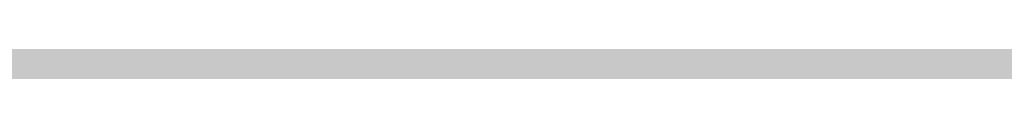
# Model space of a CAD drawing. Units: inches. Extents: x 2083 to 3317, y 1141 to 2115.
# Tile 151 of 256: x 3126.946713 to 3126.955939, y 1263.261503 to 1263.261646. Entities that reach past the tile are written whole.
import ezdxf

# ---------------------------------------------------------------- set-up
doc = ezdxf.new("R2010")
doc.units = ezdxf.units.IN
doc.layers.add('A-ANNO-DIMS', color=2, linetype='Continuous', lineweight=18)
doc.layers.add('A-WALL-PATT', color=251, linetype='Continuous', lineweight=13, true_color=0x636466)
doc.styles.get("Standard").update_dxf_attribs({"font": 'arial.ttf'})
doc.dimstyles.new('ISO-25', dxfattribs={"dimtxt": 12, "dimasz": 12, "dimexe": 1.25, "dimexo": 0.625, "dimtad": 1, "dimlunit": 3, "dimtxsty": 'Standard', "dimcen": 2.5, "dimadec": 0, "dimazin": 0, "dimtfac": 1, "dimtmove": 0, "dimatfit": 3, "dimfxl": 1, "dimarcsym": 0})

# ---------------------------------------------------------------- blocks, each defined once
blk = doc.blocks.new('*D26')
at = {"layer": 'A-ANNO-DIMS', "color": 0, "lineweight": -2, "transparency": 16777216}
for p, q in [((3088.985844, 1274.915092), (3088.985844, 1270.9519631)), ((3111.2400366, 1274.915092), (3111.2400366, 1270.9519631)), ((3076.985844, 1272.2019631), (2840.262447, 1272.2019631)), ((3111.2400366, 1272.2019631), (3088.985844, 1272.2019631)), ((3123.2400366, 1272.2019631), (3135.2400366, 1272.2019631))]:
    blk.add_line(p, q, dxfattribs=at)
at = {"layer": 'A-ANNO-DIMS', "color": 0, "transparency": 16777216}
for points in [[(3076.985844, 1274.2019631), (3076.985844, 1270.2019631), (3088.985844, 1272.2019631)], [(3123.2400366, 1274.2019631), (3123.2400366, 1270.2019631), (3111.2400366, 1272.2019631)]]:
    blk.add_solid(points, dxfattribs=at)
at = {"layer": 'Defpoints', "color": 0, "transparency": 16777216}
for p in [(3088.985844, 1275.540092), (3111.2400366, 1275.540092), (3088.985844, 1272.2019631)]:
    blk.add_point(p, dxfattribs=at)
at = {"layer": 'A-ANNO-DIMS', "color": 0, "transparency": 16777216, "insert": (2952.6241455, 1279.0316016), "char_height": 12, "attachment_point": 5}
blk.add_mtext('NIGHTSTAND 1\'-10 1/2" TYP.', dxfattribs=at)

msp = doc.modelspace()

# ---------------------------------------------------------------- hatches: boundary and pattern name
at = {"layer": 'A-WALL-PATT'}
h = msp.add_hatch(color=256, dxfattribs=at)
h.dxf.hatch_style = 1
h.paths.add_polyline_path([(3126.9597832, 2020.7613601), (2748.9597832, 2020.7613601), (2604.9597832, 2020.7613601), (2226.9597832, 2020.7613601), (2226.9597832, 1702.7613601), (2466.9597832, 1702.7613601), (2466.9597832, 1582.7613601), (2418.9597832, 1582.7613601), (2418.9597832, 1477.7613601), (2226.9597832, 1477.7613601), (2226.9597832, 1263.2613601), (2544.9597832, 1263.2613601), (2544.9597832, 1411.7613601), (2604.9597832, 1411.7613601), (2685.9597832, 1411.7613601), (2685.9597832, 1420.7613601), (2604.9597832, 1420.7613601), (2604.9597832, 1573.7613601), (2604.9597832, 1702.7613601), (2604.9597832, 2011.7613601), (2748.9597832, 2011.7613601), (2748.9597832, 1702.7613601), (2862.9597832, 1702.7613601), (2862.9597832, 1621.7613601), (2871.9597832, 1621.7613601), (2871.9597832, 1702.7613601), (2883.9597832, 1702.7613601), (2883.9597832, 1706.9394595, -0.026459), (2883.9597832, 1711.7613601), (2757.9597832, 1711.7613601), (2757.9597832, 1807.7613601), (2787.9597832, 1807.7613601), (2787.9597832, 1812.2613601), (2757.9597832, 1812.2613601), (2757.9597832, 2011.7613601), (2877.9597832, 2011.7613601), (2877.9597832, 1812.2613601), (2847.9597832, 1812.2613601), (2847.9597832, 1807.7613601), (2889.8357425, 1807.7613601), (2889.8357425, 1812.2613601), (2882.4597832, 1812.2613601), (2882.4597832, 2011.7613601), (3117.9597832, 2011.7613601), (3117.9597832, 1812.2613601), (2937.8357425, 1812.2613601), (2937.8357425, 1807.7613601), (2995.7097832, 1807.7613601), (2995.7097832, 1796.1176655), (3000.2097832, 1796.1176655), (3000.2097832, 1807.7613601), (3117.9597832, 1807.7613601), (3117.9597832, 1711.7613601), (3000.2097832, 1711.7613601), (3000.2097832, 1760.1176655), (2998.5727047, 1760.1176655, -0.020711), (2995.7097832, 1760.1176655), (2995.7097832, 1711.7613601), (2931.9597832, 1711.7613601), (2931.9597832, 1702.7613601), (3126.9597832, 1702.7613601)])
h.paths.add_polyline_path([(2471.4597832, 2011.7613601), (2471.4597832, 1810.0113601), (2462.7169357, 1810.0113601), (2462.7169357, 1805.5113601), (2505.9597832, 1805.5113601), (2505.9597832, 1810.0113601), (2475.9597832, 1810.0113601), (2475.9597832, 2011.7613601), (2595.9597832, 2011.7613601), (2595.9597832, 1810.0113601), (2565.9597832, 1810.0113601), (2565.9597832, 1805.5113601), (2595.9597832, 1805.5113601), (2595.9597832, 1711.7613601), (2235.9597832, 1711.7613601), (2235.9597832, 1805.5113601), (2353.7097832, 1805.5113601), (2353.7097832, 1796.0541624), (2358.2097832, 1796.0541624), (2358.2097832, 1805.5113601), (2414.7169357, 1805.5113601), (2414.7169357, 1810.0113601), (2235.9597832, 1810.0113601), (2235.9597832, 2011.7613601)], flags=16)
h.paths.add_polyline_path([(2270.2047343, 1994.6100082), (2270.2047343, 1970.6100082), (2246.2047343, 1970.6100082), (2246.2047343, 1994.6100082)], flags=0)
edge = h.paths.add_edge_path(flags=0)
edge.add_ellipse((2332.027391, 1899.7981761), major_axis=(-3.0429938, 3.0429938), ratio=0.16825245, start_angle=-161.3321656, end_angle=-156.3071136, ccw=False)
edge.add_ellipse((2333.0820373, 1898.7435297), major_axis=(-1.0546463, 1.0546463), ratio=0.453532097, start_angle=-123.371019, end_angle=-94.1591066)
edge = h.paths.add_edge_path(flags=0)
edge.add_ellipse((2332.027391, 1968.8762897), major_axis=(3.0429938, 3.0429938), ratio=0.16825245, start_angle=18.6678344, end_angle=23.6928864)
edge.add_spline(control_points=[(2332.9255964, 1970.6911045), (2332.2267681, 1970.3360997), (2330.8937087, 1969.6589054), (2328.4130803, 1970.9321376), (2327.2039345, 1967.7487119), (2324.7095965, 1969.9555886), (2322.5328223, 1967.012354), (2320.0128462, 1971.2958124), (2317.6803077, 1968.1578449), (2316.0405263, 1967.1020468), (2315.4269045, 1966.8096022)], knot_values=[0, 0, 0, 0, 2.267059, 4.324559, 6.685584, 8.878641, 11.121502, 14.300359, 17.755284, 19.732645, 19.732645, 19.732645, 19.732645], degree=3, periodic=0)
edge.add_ellipse((2332.027391, 1968.8762897), major_axis=(3.0429938, 3.0429938), ratio=0.16825245, start_angle=18.6678344, end_angle=23.6928864, ccw=False)
edge.add_ellipse((2333.0820373, 1969.930936), major_axis=(1.0546463, 1.0546463), ratio=0.453532097, start_angle=56.628981, end_angle=85.8408934, ccw=False)
edge = h.paths.add_edge_path(flags=0)
edge.add_spline(control_points=[(2296.4282874, 1967.9879081), (2293.6278045, 1965.3363137), (2287.7036238, 1959.727094), (2299.7438601, 1949.9956993), (2294.5325909, 1935.6685275), (2290.5732281, 1920.6035119), (2293.3941244, 1909.9736911), (2296.1854073, 1904.9665431)], knot_values=[0.099185, 0.099185, 0.099185, 0.099185, 0.345301, 0.619822, 0.982653, 1.386093, 1.810555, 1.810555, 1.810555, 1.810555], degree=3, periodic=0)
edge.add_spline(control_points=[(2296.1854073, 1904.9665431), (2297.3835817, 1902.6193002), (2298.0009694, 1901.9493116), (2298.5529698, 1901.4681549)], knot_values=[0.006246, 0.006246, 0.006246, 0.006246, 0.055476, 0.055476, 0.055476, 0.055476], degree=3, periodic=0)
edge.add_spline(control_points=[(2298.5529698, 1901.4681549), (2297.2586121, 1900.9232238), (2295.2252939, 1900.2321257), (2293.0602287, 1900.6142053), (2292.1014227, 1900.788415), (2292.0895776, 1900.790568)], knot_values=[0.312835, 0.312835, 0.312835, 0.312835, 0.40178, 0.474987, 0.475903, 0.475903, 0.475903, 0.475903], degree=3, periodic=0)
edge.add_arc((2292.7936464, 1904.6641088), 3.9370079, 215.4208969, 259.6981795, ccw=False)
edge.add_spline(control_points=[(2289.5853139, 1902.3823039), (2289.4766524, 1902.5350874), (2289.3684805, 1902.6880353), (2289.2608648, 1902.8411699)], knot_values=[0.102872, 0.102872, 0.102872, 0.102872, 0.116896, 0.116896, 0.116896, 0.116896], degree=3, periodic=0)
edge.add_spline(control_points=[(2289.2608648, 1902.8411699), (2288.6866042, 1902.5501922), (2287.6400477, 1902.0199025), (2285.8813368, 1901.8739536), (2283.8529717, 1901.5043521), (2281.7199871, 1899.7105375), (2278.4669913, 1899.492942), (2276.1571361, 1901.8832022), (2272.2589526, 1899.8040711), (2267.7776054, 1901.8431828), (2262.2438819, 1900.1840326), (2257.414927, 1901.7820606), (2254.318374, 1900.7261196), (2253.1782849, 1900.3373431)], knot_values=[0, 0, 0, 0, 1.907977, 3.477176, 5.261074, 7.972851, 11.680248, 13.717921, 16.939592, 22.789562, 27.502503, 33.595215, 37.145618, 37.145618, 37.145618, 37.145618], degree=3, periodic=0)
edge.add_line((2253.1782849, 1900.3373431), (2250.2442397, 1902.8411699))
edge.add_line((2250.2442397, 1902.8411699), (2250.2442397, 1965.8332959))
edge.add_line((2250.2442397, 1965.8332959), (2253.1782849, 1968.3371226))
edge.add_spline(control_points=[(2253.1782849, 1968.3371226), (2254.318374, 1967.9483462), (2257.414927, 1966.8924051), (2262.2438819, 1968.4904332), (2267.7776054, 1966.8312829), (2271.5267301, 1968.5372172), (2273.8759143, 1967.8282895), (2274.2067012, 1967.7276424)], knot_values=[0, 0, 0, 0, 0.09018, 0.244935, 0.364644, 0.513233, 0.537855, 0.537855, 0.537855, 0.537855], degree=3, periodic=0)
edge.add_arc((2274.3528869, 1963.7933495), 3.9370079, 72.0511336, 92.1279492, ccw=False)
edge.add_arc((2281.2969331, 1985.2300027), 18.5962982, 252.05113361, 288.56572166)
edge.add_arc((2292.3167172, 1956.0288805), 12.6460805, 71.02678788, 113.77821843, ccw=False)
edge = h.paths.add_edge_path(flags=0)
edge.add_spline(control_points=[(2274.8994147, 1951.8561946), (2275.066156, 1951.6165924), (2275.2326866, 1951.3765878), (2275.3979871, 1951.1358545)], knot_values=[1.409916, 1.409916, 1.409916, 1.409916, 1.43159, 1.43159, 1.43159, 1.43159], degree=3, periodic=0)
edge.add_spline(control_points=[(2275.3979871, 1951.1358545), (2275.7921055, 1950.5618854), (2276.1792311, 1949.9837745), (2276.5455462, 1949.3971029)], knot_values=[1.358238, 1.358238, 1.358238, 1.358238, 1.409916, 1.409916, 1.409916, 1.409916], degree=3, periodic=0)
edge.add_line((2276.5455462, 1949.3971029), (2277.437289, 1947.8621847))
edge.add_spline(control_points=[(2277.437289, 1947.8621847), (2276.3038341, 1945.6731147), (2274.6396979, 1942.4268817), (2274.631615, 1938.0938998), (2272.7991237, 1930.8515498), (2274.3564261, 1943.8970461), (2275.9476814, 1947.9233558), (2276.5455462, 1949.3971029)], knot_values=[0.005632, 0.005632, 0.005632, 0.005632, 0.186014, 0.266002, 0.357087, 0.59639, 0.739732, 0.739732, 0.739732, 0.739732], degree=3, periodic=0)
edge.add_spline(control_points=[(2276.5455462, 1949.3971029), (2276.1792311, 1949.9837745), (2275.7921055, 1950.5618854), (2275.3979871, 1951.1358545)], knot_values=[1.358238, 1.358238, 1.358238, 1.358238, 1.409916, 1.409916, 1.409916, 1.409916], degree=3, periodic=0)
edge.add_spline(control_points=[(2275.3979871, 1951.1358545), (2274.9425002, 1950.0804523), (2274.2077604, 1948.0252718), (2273.9346018, 1944.8514774), (2272.4685341, 1937.6274891), (2273.4662155, 1945.6964663), (2274.7006154, 1951.0594725), (2274.8994147, 1951.8561946)], knot_values=[0.104364, 0.104364, 0.104364, 0.104364, 0.189636, 0.269624, 0.36071, 0.600013, 0.644622, 0.644622, 0.644622, 0.644622], degree=3, periodic=0)
h.paths.add_polyline_path([(2269.1675139, 1963.1275729, -0.357527), (2268.170633, 1960.9763695, -0.092561), (2268.170633, 1939.4363249, -0.357527), (2269.1675139, 1937.2851215, -0.357527), (2267.0163105, 1938.2820024, -0.164785), (2254.6855813, 1938.2820024, -0.357527), (2252.5343779, 1937.2851215, -0.357527), (2253.5312587, 1939.4363249, -0.092561), (2253.5312587, 1960.9763695, -0.357527), (2252.5343779, 1963.1275729, -0.357527), (2254.6855813, 1962.130692, -0.164785), (2267.0163105, 1962.130692, -0.357527)], flags=0)
h.paths.add_polyline_path([(2248.8740679, 1967.8017998), (2248.8740679, 1957.0277095), (2249.4577833, 1957.0277095), (2249.4577833, 1911.6467562), (2248.8740679, 1911.6467562), (2248.8740679, 1900.8726659), (2246.5118632, 1900.8726659, 0.197327), (2244.1496584, 1902.4568734), (2244.1496584, 1966.2175923, 0.197327), (2246.5118632, 1967.8017998)], flags=0)
h.paths.add_polyline_path([(2269.1675139, 1931.3893442, -0.357527), (2268.170633, 1929.2381408, -0.092561), (2268.170633, 1907.6980962, -0.357527), (2269.1675139, 1905.5468928, -0.357527), (2267.0163105, 1906.5437737, -0.164785), (2254.6855813, 1906.5437737, -0.357527), (2252.5343779, 1905.5468928, -0.357527), (2253.5312587, 1907.6980962, -0.092561), (2253.5312587, 1929.2381408, -0.357527), (2252.5343779, 1931.3893442, -0.357527), (2254.6855813, 1930.3924634, -0.164785), (2267.0163105, 1930.3924634, -0.357527)], flags=0)
edge = h.paths.add_edge_path(flags=0)
edge.add_spline(control_points=[(2276.1968578, 1906.7237016), (2276.1681442, 1909.0289278), (2276.1140492, 1913.371852), (2270.5984171, 1924.9249783), (2273.9051746, 1919.0127787), (2275.9217115, 1916.2620626), (2275.4745699, 1912.4021495), (2277.2578735, 1910.3806206), (2276.6960436, 1908.2250358), (2276.6462176, 1906.8130226), (2276.6178249, 1906.0084068)], knot_values=[0, 0, 0, 0, 8.61026, 16.221274, 18.843057, 23.804898, 27.440828, 29.356102, 31.203478, 33.650687, 33.650687, 33.650687, 33.650687], degree=3, periodic=0)
edge.add_spline(control_points=[(2276.6178249, 1906.0084068), (2276.6233131, 1905.6241436), (2276.4977381, 1904.6286608), (2275.4417789, 1903.8547251), (2274.9373144, 1903.0804497), (2274.8590804, 1902.8411699)], knot_values=[0.156488, 0.156488, 0.156488, 0.156488, 0.184398, 0.231376, 0.250598, 0.250598, 0.250598, 0.250598], degree=3, periodic=0)
edge.add_line((2274.8590804, 1902.8411699), (2276.50598, 1902.8411699))
edge.add_spline(control_points=[(2276.50598, 1902.8411699), (2276.7883084, 1903.0849395), (2277.6650711, 1904.1251958), (2278.2495378, 1904.340738), (2277.6538719, 1908.5273866), (2278.15567, 1906.2278078), (2278.100464, 1905.2859484), (2278.8466748, 1904.0690054), (2277.8567853, 1903.4149482), (2277.8741909, 1902.9910497), (2277.9035616, 1902.8411699)], knot_values=[0.059574, 0.059574, 0.059574, 0.059574, 0.080753, 0.103741, 0.16972, 0.176036, 0.207137, 0.240474, 0.262341, 0.27366, 0.27366, 0.27366, 0.27366], degree=3, periodic=0)
edge.add_line((2277.9035616, 1902.8411699), (2280.0298255, 1902.8411699))
edge.add_spline(control_points=[(2280.0298255, 1902.8411699), (2279.8882214, 1903.088398), (2279.4992571, 1903.9815512), (2280.1522839, 1905.9393491), (2278.103615, 1909.6577572), (2279.7623946, 1907.185285), (2280.3279002, 1904.8748608), (2280.4851086, 1903.4895904), (2281.4632687, 1903.2494323), (2281.7583431, 1902.9364967), (2281.8340361, 1902.8411699)], knot_values=[0.013856, 0.013856, 0.013856, 0.013856, 0.034874, 0.088867, 0.107879, 0.126738, 0.158714, 0.193757, 0.217487, 0.226722, 0.226722, 0.226722, 0.226722], degree=3, periodic=0)
edge.add_spline(control_points=[(2281.8340361, 1902.8411699), (2281.7875348, 1902.8267029), (2281.6470224, 1902.7829881), (2281.3955272, 1902.85949), (2281.088077, 1902.9852418), (2280.7206826, 1903.060902), (2280.3334513, 1903.0257257), (2280.1247668, 1902.898879), (2280.0298255, 1902.8411699)], knot_values=[0, 0, 0, 0, 0.14413, 0.435517, 0.749276, 1.153046, 1.548371, 1.878348, 1.878348, 1.878348, 1.878348], degree=3, periodic=0)
edge.add_line((2280.0298255, 1902.8411699), (2277.9035616, 1902.8411699))
edge.add_spline(control_points=[(2277.9035616, 1902.8411699), (2277.892855, 1902.7958553), (2277.865396, 1902.6796374), (2277.6074793, 1902.6874828), (2277.2740503, 1902.8006999), (2276.8379209, 1902.6197745), (2276.5838074, 1902.7892611), (2276.50598, 1902.8411699)], knot_values=[0, 0, 0, 0, 0.127189, 0.326199, 0.628009, 1.24357, 1.515331, 1.515331, 1.515331, 1.515331], degree=3, periodic=0)
edge.add_line((2276.50598, 1902.8411699), (2274.8590804, 1902.8411699))
edge.add_spline(control_points=[(2274.8590804, 1902.8411699), (2274.8144367, 1902.8985868), (2274.7251297, 1903.013446), (2274.4934765, 1903.1189684), (2274.2442854, 1902.9605386), (2273.9371207, 1903.1849416), (2273.6140395, 1902.9831428), (2273.4083164, 1902.8830449), (2273.322254, 1902.8411699)], knot_values=[0, 0, 0, 0, 0.21843, 0.436957, 0.687977, 0.990379, 1.398396, 1.69185, 1.69185, 1.69185, 1.69185], degree=3, periodic=0)
edge.add_spline(control_points=[(2273.322254, 1902.8411699), (2273.6167403, 1903.445692), (2274.2739977, 1904.5382529), (2276.0272387, 1904.5737017), (2276.2069634, 1906.5836372), (2276.1968578, 1906.7237016)], knot_values=[0.012227, 0.012227, 0.012227, 0.012227, 0.059472, 0.106218, 0.134458, 0.134458, 0.134458, 0.134458], degree=3, periodic=0)
h.paths.add_polyline_path([(2270.7760538, 1897.7898284), (2270.7760538, 1873.7898284), (2246.7760538, 1873.7898284), (2246.7760538, 1897.7898284)], flags=0)
h.paths.add_polyline_path([(2353.7097832, 1760.0050593), (2353.7097832, 1760.0541624), (2358.2097832, 1760.0541624, -0.033729)], flags=0)
h.paths.add_polyline_path([(2321.8191188, 1737.5291862), (2341.9953271, 1737.5291862, -0.414214), (2343.2032727, 1736.3212406), (2343.2032727, 1721.0205964, -0.414214), (2341.9953271, 1719.8126508), (2321.8191188, 1719.8126508, -0.414214), (2320.6111732, 1721.0205964), (2320.6111732, 1736.3212406, -0.414214)], flags=0)
h.paths.add_polyline_path([(2324.2350099, 1736.3212406), (2339.5794359, 1736.3212406, -0.414214), (2341.9953271, 1733.9053494), (2341.9953271, 1725.4497302, -0.414214), (2339.5794359, 1723.033839), (2333.6805885, 1723.033839), (2333.8453172, 1722.0454666, -0.870646), (2335.4253988, 1721.8258934, -0.767327), (2333.922694, 1721.4232449), (2331.2910241, 1721.4232449, -0.767327), (2329.7883193, 1721.8258934, -0.870646), (2331.3684009, 1722.0454666), (2331.5331296, 1723.033839), (2324.2350099, 1723.033839, -0.414214), (2321.8191188, 1725.4497302), (2321.8191188, 1733.9053494, -0.414214)], flags=0)
h.paths.add_polyline_path([(2570.4837892, 1928.6154443), (2589.6837892, 1928.6154443), (2590.1688286, 1928.6154443), (2590.1688286, 1904.9933971), (2570.4837892, 1904.9933971)], flags=0)
h.paths.add_polyline_path([(2574.4473242, 1927.2638215, -1), (2572.8288357, 1927.2638215, -1)], flags=0)
h.paths.add_polyline_path([(2573.0898665, 1926.9408768), (2573.925032, 1927.7760423), (2574.1477428, 1927.5533315), (2573.3125773, 1926.718166)], flags=0)
h.paths.add_polyline_path([(2578.7790648, 1919.7296175, -1), (2571.5916632, 1919.7296175, -1)], flags=0)
h.paths.add_polyline_path([(2578.385364, 1919.7296175, -1), (2571.985364, 1919.7296175, -1)], flags=0)
h.paths.add_polyline_path([(2331.5957638, 1729.4762156, -1), (2333.6179542, 1729.4762156, -1)], flags=0)
h.paths.add_polyline_path([(2578.0342282, 1927.2638215, -1), (2576.4157396, 1927.2638215, -1)], flags=0)
h.paths.add_polyline_path([(2576.6888513, 1927.5310886), (2576.9115621, 1927.7537993), (2577.7467276, 1926.9186339), (2577.5240168, 1926.6959231)], flags=0)
h.paths.add_polyline_path([(2578.1390648, 1909.8595388, -1), (2572.2316632, 1909.8595388, -1)], flags=0)
h.paths.add_polyline_path([(2577.745364, 1909.8595388, -1), (2572.625364, 1909.8595388, -1)], flags=0)
h.paths.add_polyline_path([(2583.7977179, 1927.2638215, -1), (2582.1792294, 1927.2638215, -1)], flags=0)
h.paths.add_polyline_path([(2582.7186487, 1927.7537993), (2583.5538142, 1926.9186339), (2583.3311034, 1926.6959231), (2582.4959379, 1927.5310886)], flags=0)
h.paths.add_polyline_path([(2582.4959379, 1927.5310886), (2582.7186487, 1927.7537993), (2583.5538142, 1926.9186339), (2583.3311034, 1926.6959231)], flags=0)
h.paths.add_polyline_path([(2587.7390648, 1920.5296175, -1), (2581.8316632, 1920.5296175, -1)], flags=0)
h.paths.add_polyline_path([(2587.345364, 1920.5296175, -1), (2582.225364, 1920.5296175, -1)], flags=0)
h.paths.add_polyline_path([(2587.3846219, 1927.2638215, -1), (2585.7661333, 1927.2638215, -1)], flags=0)
h.paths.add_polyline_path([(2586.0819925, 1926.9802469), (2586.917158, 1927.8154124), (2587.1398688, 1927.5927016), (2586.3047033, 1926.7575361)], flags=0)
h.paths.add_polyline_path([(2588.3790648, 1910.6595388, -1), (2581.1916632, 1910.6595388, -1)], flags=0)
h.paths.add_polyline_path([(2587.985364, 1910.6595388, -1), (2581.585364, 1910.6595388, -1)], flags=0)
h.paths.add_polyline_path([(2417.1677288, 1729.4778955), (2437.3439372, 1729.4778955, -0.414214), (2438.5518828, 1728.2699499), (2438.5518828, 1712.9693057, -0.414214), (2437.3439372, 1711.7613601), (2417.1677288, 1711.7613601, -0.414214), (2415.9597832, 1712.9693057), (2415.9597832, 1728.2699499, -0.414214)], flags=0)
h.paths.add_polyline_path([(2419.58362, 1728.2699499), (2434.928046, 1728.2699499, -0.414214), (2437.3439372, 1725.8540587), (2437.3439372, 1717.3984395, -0.414214), (2434.928046, 1714.9825483), (2429.0291985, 1714.9825483), (2429.1939273, 1713.9941758, -0.870646), (2430.7740089, 1713.7746027, -0.767327), (2429.2713041, 1713.3719542), (2426.6396342, 1713.3719542, -0.767327), (2425.1369294, 1713.7746027, -0.870646), (2426.717011, 1713.9941758), (2426.8817397, 1714.9825483), (2419.58362, 1714.9825483, -0.414214), (2417.1677288, 1717.3984395), (2417.1677288, 1725.8540587, -0.414214)], flags=0)
h.paths.add_polyline_path([(2419.58362, 1728.2699499), (2434.928046, 1728.2699499, -0.414214), (2437.3439372, 1725.8540587), (2437.3439372, 1717.3984395, -0.414214), (2434.928046, 1714.9825483), (2429.0291985, 1714.9825483), (2428.3581177, 1719.0090337), (2427.5528206, 1719.0090337), (2426.8817397, 1714.9825483), (2419.58362, 1714.9825483, -0.414214), (2417.1677288, 1717.3984395), (2417.1677288, 1725.8540587, -0.414214)], flags=0)
h.paths.add_polyline_path([(2426.9443739, 1721.4249248, -1), (2428.9665643, 1721.4249248, -1)], flags=0)
h.paths.add_polyline_path([(2475.9597832, 1702.7613601), (2595.9597832, 1702.7613601), (2595.9597832, 1582.7613601), (2475.9597832, 1582.7613601)], flags=16)
h.paths.add_polyline_path([(2427.9597832, 1573.7613601), (2595.9597832, 1573.7613601), (2595.9597832, 1468.7613601), (2595.9597832, 1420.7613601), (2384.4597832, 1420.7613601), (2384.4597832, 1468.7613601), (2427.9597832, 1468.7613601)], flags=16)
h.paths.add_polyline_path([(2379.9597832, 1468.7613601), (2379.9597832, 1420.7613601), (2235.9597832, 1420.7613601), (2235.9597832, 1468.7613601)], flags=16)
h.paths.add_polyline_path([(2317.8159962, 1466.695767), (2337.9922045, 1466.695767, -0.414214), (2339.2001501, 1465.4878214), (2339.2001501, 1450.1871771, -0.414214), (2337.9922045, 1448.9792315), (2317.8159962, 1448.9792315, -0.414214), (2316.6080506, 1450.1871771), (2316.6080506, 1465.4878214, -0.414214)], flags=0)
h.paths.add_polyline_path([(2320.2318874, 1465.4878214), (2335.5763133, 1465.4878214, -0.414214), (2337.9922045, 1463.0719302), (2337.9922045, 1454.616311, -0.414214), (2335.5763133, 1452.2004198), (2329.6774659, 1452.2004198), (2329.8421946, 1451.2120473, -0.870646), (2331.4222762, 1450.9924742, -0.767327), (2329.9195714, 1450.5898257), (2327.2879015, 1450.5898257, -0.767327), (2325.7851967, 1450.9924742, -0.870646), (2327.3652783, 1451.2120473), (2327.530007, 1452.2004198), (2320.2318874, 1452.2004198, -0.414214), (2317.8159962, 1454.616311), (2317.8159962, 1463.0719302, -0.414214)], flags=0)
h.paths.add_polyline_path([(2320.2318874, 1465.4878214), (2335.5763133, 1465.4878214, -0.414214), (2337.9922045, 1463.0719302), (2337.9922045, 1454.616311, -0.414214), (2335.5763133, 1452.2004198), (2329.6774659, 1452.2004198), (2329.006385, 1456.2269051), (2328.2010879, 1456.2269051), (2327.530007, 1452.2004198), (2320.2318874, 1452.2004198, -0.414214), (2317.8159962, 1454.616311), (2317.8159962, 1463.0719302, -0.414214)], flags=0)
h.paths.add_polyline_path([(2327.5926413, 1458.6427963, -1), (2329.6148317, 1458.6427963, -1)], flags=0)
h.paths.add_polyline_path([(2244.4117436, 1433.3404531), (2241.9209449, 1433.3404531, -0.414214), (2240.0178562, 1435.2435418), (2240.0178562, 1440.9528078, -0.414211), (2241.920925, 1442.8558965), (2244.4117436, 1442.8558965, -1.976472)], flags=0)
h.paths.add_polyline_path([(2245.3568884, 1434.3975358, -0.414214), (2245.3568884, 1441.7988138, -2.144098)], flags=0)
h.paths.add_polyline_path([(2535.9597832, 1416.2613601), (2535.9597832, 1272.2613601), (2235.9597832, 1272.2613601), (2235.9597832, 1416.2613601)], flags=16)
h.paths.add_polyline_path([(2260.1195614, 1384.2928413), (2260.1195614, 1362.0386487), (2237.8653688, 1362.0386487), (2237.8653688, 1384.2928413)], flags=0)
edge = h.paths.add_edge_path(flags=0)
edge.add_line((2318.2518466, 1362.0932983), (2318.1457968, 1362.0009726))
edge.add_ellipse((2317.4451158, 1360.4310442), major_axis=(2.8216404, 2.8216404), ratio=0.16825245, start_angle=18.6678344, end_angle=20.9481273, ccw=False)
edge.add_ellipse((2318.4230451, 1361.4089735), major_axis=(0.9779293, 0.9779293), ratio=0.453532097, start_angle=56.628981, end_angle=70.2262012, ccw=False)
edge = h.paths.add_edge_path(flags=0)
edge.add_line((2319.1073699, 1295.5710784), (2319.0150442, 1295.6771282))
edge.add_ellipse((2317.4451158, 1296.3778091), major_axis=(-2.8216404, 2.8216404), ratio=0.16825245, start_angle=-161.3321656, end_angle=-159.0518727, ccw=False)
edge.add_ellipse((2318.4230451, 1295.3998798), major_axis=(-0.9779293, 0.9779293), ratio=0.453532097, start_angle=-123.371019, end_angle=-109.7737988)
edge = h.paths.add_edge_path(flags=0)
edge.add_spline(control_points=[(2284.2103489, 1301.1702189), (2284.5806878, 1300.444719), (2284.8911891, 1299.8920243), (2285.159553, 1299.4610182)], knot_values=[0.039066, 0.039066, 0.039066, 0.039066, 0.055476, 0.055476, 0.055476, 0.055476], degree=3, periodic=0)
edge.add_line((2285.159553, 1299.4610182), (2284.2103489, 1301.1702189))
edge = h.paths.add_edge_path(flags=0)
edge.add_line((2280.4124579, 1297.2980125), (2283.3699905, 1297.0361216))
edge.add_line((2283.3699905, 1297.0361216), (2286.4056902, 1297.9263104))
edge.add_spline(control_points=[(2286.4056902, 1297.9263104), (2285.305487, 1297.4631193), (2284.3447774, 1297.1291508), (2283.3699905, 1297.0361216)], knot_values=[0.394369, 0.394369, 0.394369, 0.394369, 0.475903, 0.475903, 0.475903, 0.475903], degree=3, periodic=0)
edge.add_spline(control_points=[(2283.3699905, 1297.0361216), (2283.2813895, 1297.027666), (2282.316289, 1296.9573356), (2281.3125019, 1297.1344787), (2280.4234414, 1297.2960161), (2280.4124579, 1297.2980125)], knot_values=[0.312835, 0.312835, 0.312835, 0.312835, 0.320246, 0.393453, 0.394369, 0.394369, 0.394369, 0.394369], degree=3, periodic=0)
edge = h.paths.add_edge_path(flags=0)
edge.add_line((2284.4355615, 1359.6072854), (2280.4462909, 1355.328047))
edge.add_line((2280.4462909, 1355.328047), (2279.5799868, 1351.0177544))
edge.add_line((2279.5799868, 1351.0177544), (2282.4129737, 1346.5804327))
edge.add_spline(control_points=[(2282.4129737, 1346.5804327), (2283.1533308, 1345.5892358), (2284.2528957, 1344.0288973), (2284.801037, 1342.3871671), (2284.9351625, 1341.8055443)], knot_values=[1.240098, 1.240098, 1.240098, 1.240098, 1.332892, 1.382712, 1.382712, 1.382712, 1.382712], degree=3, periodic=0)
edge.add_spline(control_points=[(2284.9351625, 1341.8055443), (2285.3191079, 1340.1406002), (2285.2330291, 1338.4092041), (2284.9099384, 1336.6541222)], knot_values=[1.097484, 1.097484, 1.097484, 1.097484, 1.240098, 1.240098, 1.240098, 1.240098], degree=3, periodic=0)
edge.add_spline(control_points=[(2284.9099384, 1336.6541222), (2284.5868478, 1334.8990403), (2284.0267453, 1333.1202725), (2283.4626437, 1331.3605849)], knot_values=[0.95487, 0.95487, 0.95487, 0.95487, 1.097484, 1.097484, 1.097484, 1.097484], degree=3, periodic=0)
edge.add_line((2283.4626437, 1331.3605849), (2281.8903759, 1326.153357))
edge.add_line((2281.8903759, 1326.153357), (2280.7562592, 1321.0560888))
edge.add_line((2280.7562592, 1321.0560888), (2280.2992048, 1316.0019772))
edge.add_line((2280.2992048, 1316.0019772), (2280.7159327, 1310.9500678))
edge.add_line((2280.7159327, 1310.9500678), (2282.0280939, 1305.9721367))
edge.add_line((2282.0280939, 1305.9721367), (2284.2103489, 1301.1702189))
edge.add_spline(control_points=[(2284.2103489, 1301.1702189), (2283.3407305, 1302.7301854), (2282.6119044, 1304.3364933), (2282.0280939, 1305.9721367)], knot_values=[0.099185, 0.099185, 0.099185, 0.099185, 0.241799, 0.241799, 0.241799, 0.241799], degree=3, periodic=0)
edge.add_spline(control_points=[(2282.0280939, 1305.9721367), (2281.4442835, 1307.6077801), (2281.0054886, 1309.2727591), (2280.7159327, 1310.9500678)], knot_values=[0.241799, 0.241799, 0.241799, 0.241799, 0.384413, 0.384413, 0.384413, 0.384413], degree=3, periodic=0)
edge.add_spline(control_points=[(2280.7159327, 1310.9500678), (2280.4332411, 1312.5876134), (2280.2893863, 1314.2769594), (2280.2988938, 1315.9620324), (2280.2992048, 1316.0019772)], knot_values=[0.384413, 0.384413, 0.384413, 0.384413, 0.523647, 0.527028, 0.527028, 0.527028, 0.527028], degree=3, periodic=0)
edge.add_spline(control_points=[(2280.2992048, 1316.0019772), (2280.3123257, 1317.6869552), (2280.4778706, 1319.3679256), (2280.7562592, 1321.0560888)], knot_values=[0.527028, 0.527028, 0.527028, 0.527028, 0.669642, 0.669642, 0.669642, 0.669642], degree=3, periodic=0)
edge.add_spline(control_points=[(2280.7562592, 1321.0560888), (2281.0346478, 1322.7442519), (2281.4258801, 1324.4396079), (2281.8903759, 1326.153357)], knot_values=[0.669642, 0.669642, 0.669642, 0.669642, 0.812256, 0.812256, 0.812256, 0.812256], degree=3, periodic=0)
edge.add_spline(control_points=[(2281.8903759, 1326.153357), (2282.2643834, 1327.5332507), (2282.7878702, 1329.2618097), (2283.352751, 1331.0177803), (2283.4626437, 1331.3605849)], knot_values=[0.812256, 0.812256, 0.812256, 0.812256, 0.927087, 0.95487, 0.95487, 0.95487, 0.95487], degree=3, periodic=0)
edge.add_line((2283.4626437, 1331.3605849), (2284.9099384, 1336.6541222))
edge.add_line((2284.9099384, 1336.6541222), (2284.9351625, 1341.8055443))
edge.add_line((2284.9351625, 1341.8055443), (2282.4129737, 1346.5804327))
edge.add_spline(control_points=[(2282.4129737, 1346.5804327), (2281.2751273, 1348.1037918), (2280.0784467, 1349.5703178), (2279.5799868, 1351.0177544)], knot_values=[1.382712, 1.382712, 1.382712, 1.382712, 1.525326, 1.525326, 1.525326, 1.525326], degree=3, periodic=0)
edge.add_spline(control_points=[(2279.5799868, 1351.0177544), (2279.4432818, 1351.4147209), (2279.1363124, 1352.856922), (2279.7351897, 1354.2903851), (2280.4462909, 1355.328047)], knot_values=[1.525326, 1.525326, 1.525326, 1.525326, 1.564439, 1.667941, 1.667941, 1.667941, 1.667941], degree=3, periodic=0)
edge.add_spline(control_points=[(2280.4462909, 1355.328047), (2281.4261132, 1356.7578354), (2282.9308373, 1358.1825604), (2284.4355615, 1359.6072854)], knot_values=[1.667941, 1.667941, 1.667941, 1.667941, 1.810555, 1.810555, 1.810555, 1.810555], degree=3, periodic=0)
edge.add_arc((2280.6230749, 1348.518181), 11.7261796, 71.02678788, 113.77821843)
edge.add_arc((2270.4048917, 1375.5951559), 17.2435667, 252.05113361, 288.56572166, ccw=False)
edge.add_arc((2263.9659692, 1355.7178471), 3.6506221, 72.0511336, 92.1279492)
edge.add_arc((2263.9659692, 1355.7178471), 3.6506221, 92.1279492, 177.98513)
edge.add_spline(control_points=[(2260.3176041, 1355.8461989), (2260.2604169, 1354.2206683), (2260.551278, 1350.1865469), (2262.9993445, 1346.7662507), (2264.4727415, 1344.6490245)], knot_values=[1.43159, 1.43159, 1.43159, 1.43159, 1.564144, 1.770695, 1.770695, 1.770695, 1.770695], degree=3, periodic=0)
edge.add_line((2264.4727415, 1344.6490245), (2264.9355904, 1343.9825301))
edge.add_spline(control_points=[(2263.8010444, 1340.2481052), (2263.8432379, 1340.5140884), (2264.0672444, 1341.7564652), (2264.5126928, 1343.0024532), (2264.9350468, 1343.9810834)], knot_values=[0.53657, 0.53657, 0.53657, 0.53657, 0.559349, 0.644622, 0.644622, 0.644622, 0.644622], degree=3, periodic=0)
edge.add_spline(control_points=[(2264.9350468, 1343.9810834), (2265.1177715, 1343.7149747), (2265.2988751, 1343.4479058), (2265.4767562, 1343.1793646)], knot_values=[1.384077, 1.384077, 1.384077, 1.384077, 1.409916, 1.409916, 1.409916, 1.409916], degree=3, periodic=0)
edge.add_spline(control_points=[(2265.4767562, 1343.1793646), (2265.6546373, 1342.9108234), (2265.8292958, 1342.64081), (2265.9991301, 1342.368812)], knot_values=[1.358238, 1.358238, 1.358238, 1.358238, 1.384077, 1.384077, 1.384077, 1.384077], degree=3, periodic=0)
edge.add_line((2265.9991301, 1342.368812), (2266.8260057, 1340.9455468))
edge.add_spline(control_points=[(2266.8260057, 1340.9455468), (2268.894401, 1337.0896912), (2271.3981727, 1325.8430009), (2270.5161644, 1310.5685568), (2275.9193759, 1301.860609), (2277.7895113, 1299.1994495)], knot_values=[0.116896, 0.116896, 0.116896, 0.116896, 0.472987, 1.050969, 1.313793, 1.313793, 1.313793, 1.313793], degree=3, periodic=0)
edge.add_spline(control_points=[(2277.7895113, 1299.1994495), (2277.8394051, 1299.1284519), (2277.8894277, 1299.0574975), (2277.9395717, 1298.9865839)], knot_values=[0.109884, 0.109884, 0.109884, 0.109884, 0.116896, 0.116896, 0.116896, 0.116896], degree=3, periodic=0)
edge.add_line((2277.9395717, 1298.9865839), (2277.7888489, 1299.1991139))
edge.add_spline(control_points=[(2277.7888489, 1299.1991139), (2277.2565819, 1298.9294144), (2276.2863504, 1298.4379024), (2275.0393517, 1298.3344186), (2274.3833299, 1298.2388951), (2274.2152543, 1298.209338)], knot_values=[33.12187, 33.12187, 33.12187, 33.12187, 35.029056, 36.598255, 37.144827, 37.144827, 37.144827, 37.144827], degree=3, periodic=0)
edge.add_line((2274.2152543, 1298.209338), (2273.073147, 1297.8929607))
edge.add_spline(control_points=[(2273.073147, 1297.8929607), (2272.3229363, 1297.579784), (2271.0391507, 1296.5105078), (2269.2483948, 1296.2260622), (2268.4231004, 1296.3746543)], knot_values=[26.532584, 26.532584, 26.532584, 26.532584, 29.198919, 31.839101, 31.839101, 31.839101, 31.839101], degree=3, periodic=0)
edge.add_line((2268.4231004, 1296.3746543), (2263.8785014, 1297.4575338))
edge.add_spline(control_points=[(2263.8785014, 1297.4575338), (2263.5560769, 1297.3594345), (2261.8603064, 1296.8386943), (2260.2387805, 1297.2824073), (2258.9334543, 1297.5164611)], knot_values=[15.919551, 15.919551, 15.919551, 15.919551, 16.939592, 21.226067, 21.226067, 21.226067, 21.226067], degree=3, periodic=0)
edge.add_line((2258.9334543, 1297.5164611), (2254.0552332, 1297.3290098))
edge.add_spline(control_points=[(2254.0552332, 1297.3290098), (2253.7555255, 1297.295815), (2252.1136834, 1297.1651738), (2250.4618687, 1297.5442209), (2249.1296862, 1297.6678818)], knot_values=[5.306517, 5.306517, 5.306517, 5.306517, 6.276435, 10.613034, 10.613034, 10.613034, 10.613034], degree=3, periodic=0)
edge.add_line((2249.1296862, 1297.6678818), (2244.3316495, 1296.8777561))
edge.add_line((2244.3316495, 1296.8777561), (2241.6110326, 1299.1994495))
edge.add_line((2241.6110326, 1299.1994495), (2241.6110326, 1357.6094038))
edge.add_line((2241.6110326, 1357.6094038), (2244.3316495, 1359.9310973))
edge.add_line((2244.3316495, 1359.9310973), (2252.7288228, 1359.5426917))
edge.add_spline(control_points=[(2252.7288228, 1359.5426917), (2252.8709387, 1359.5464396), (2253.3057402, 1359.5481716), (2253.7398447, 1359.5142744), (2254.0317419, 1359.4824261)], knot_values=[0.233291, 0.233291, 0.233291, 0.233291, 0.244935, 0.268927, 0.268927, 0.268927, 0.268927], degree=3, periodic=0)
edge.add_line((2254.0317419, 1359.4824261), (2259.5871899, 1359.4163899))
edge.add_spline(control_points=[(2259.5871899, 1359.4163899), (2260.6770676, 1359.6285026), (2262.0731971, 1359.8970025), (2263.5236925, 1359.4592776), (2263.8304173, 1359.3659518)], knot_values=[0.422516, 0.422516, 0.422516, 0.422516, 0.513233, 0.537855, 0.537855, 0.537855, 0.537855], degree=3, periodic=0)
edge.add_arc((2263.9659692, 1355.7178471), 3.6506221, 72.0511336, 92.1279492, ccw=False)
edge.add_arc((2270.4048917, 1375.5951559), 17.2435667, 252.05113361, 288.56572166)
edge.add_arc((2280.6230749, 1348.518181), 11.7261796, 71.02678788, 113.77821843, ccw=False)
h.paths.add_polyline_path([(2240.3405298, 1359.4347149), (2240.3405298, 1349.4443532), (2240.8817846, 1349.4443532), (2240.8817846, 1307.3645001), (2240.3405298, 1307.3645001), (2240.3405298, 1297.3741385), (2238.1501565, 1297.3741385, 0.197327), (2235.9597832, 1298.8431076), (2235.9597832, 1357.9657458, 0.197327), (2238.1501565, 1359.4347149)], flags=0)
h.paths.add_polyline_path([(2259.1577904, 1355.1005005, -0.357527), (2258.2334246, 1353.1057799, -0.092561), (2258.2334246, 1333.1326007, -0.357527), (2259.1577904, 1331.1378801, -0.357527), (2257.1630698, 1332.0622458, -0.164785), (2245.7293022, 1332.0622458, -0.357527), (2243.7345816, 1331.1378801, -0.357527), (2244.6589474, 1333.1326007, -0.092561), (2244.6589474, 1353.1057799, -0.357527), (2243.7345816, 1355.1005005, -0.357527), (2245.7293022, 1354.1761347, -0.164785), (2257.1630698, 1354.1761347, -0.357527)], flags=0)
edge = h.paths.add_edge_path(flags=0)
edge.add_line((2265.9991301, 1342.368812), (2266.8260057, 1340.9455468))
edge.add_line((2266.8260057, 1340.9455468), (2265.3075567, 1337.8140664))
edge.add_line((2265.3075567, 1337.8140664), (2264.358232, 1334.6529388))
edge.add_line((2264.358232, 1334.6529388), (2264.2620123, 1333.7997046))
edge.add_spline(control_points=[(2264.2620123, 1333.7997046), (2264.2083565, 1333.187055), (2264.1620602, 1332.3655252), (2264.0071444, 1331.4139326), (2263.9690487, 1331.2018338)], knot_values=[0.464444, 0.464444, 0.464444, 0.464444, 0.516691, 0.531608, 0.531608, 0.531608, 0.531608], degree=3, periodic=0)
edge.add_spline(control_points=[(2263.9690487, 1331.2018338), (2263.7745349, 1330.1188727), (2263.4243703, 1328.7908386), (2263.2574202, 1328.5306516), (2263.2340282, 1328.5146115)], knot_values=[0.372682, 0.372682, 0.372682, 0.372682, 0.44885, 0.464444, 0.464444, 0.464444, 0.464444], degree=3, periodic=0)
edge.add_spline(control_points=[(2263.2340282, 1328.5146115), (2263.096382, 1328.4202271), (2263.1311696, 1329.3014765), (2263.2749528, 1330.6157493)], knot_values=[0.280919, 0.280919, 0.280919, 0.280919, 0.372682, 0.372682, 0.372682, 0.372682], degree=3, periodic=0)
edge.add_spline(control_points=[(2263.2749528, 1330.6157493), (2263.4187361, 1331.930022), (2263.6715151, 1333.677318), (2263.9698519, 1335.3150268)], knot_values=[0.189157, 0.189157, 0.189157, 0.189157, 0.280919, 0.280919, 0.280919, 0.280919], degree=3, periodic=0)
edge.add_spline(control_points=[(2263.9698519, 1335.3150268), (2264.1004958, 1336.0321917), (2264.4187827, 1337.6219113), (2264.7548476, 1338.8644304), (2264.9474193, 1339.4911244)], knot_values=[0.097394, 0.097394, 0.097394, 0.097394, 0.137578, 0.189157, 0.189157, 0.189157, 0.189157], degree=3, periodic=0)
edge.add_spline(control_points=[(2264.9474193, 1339.4911244), (2265.2900171, 1340.6060546), (2265.6442376, 1341.4939958), (2265.9991301, 1342.368812)], knot_values=[0.005632, 0.005632, 0.005632, 0.005632, 0.097394, 0.097394, 0.097394, 0.097394], degree=3, periodic=0)
h.paths.add_polyline_path([(2259.1577904, 1325.6709733, -0.357527), (2258.2334246, 1323.6762527, -0.092561), (2258.2334246, 1303.7030735, -0.357527), (2259.1577904, 1301.7083529, -0.357527), (2257.1630698, 1302.6327186, -0.164785), (2245.7293022, 1302.6327186, -0.357527), (2243.7345816, 1301.7083529, -0.357527), (2244.6589474, 1303.7030735, -0.092561), (2244.6589474, 1323.6762527, -0.357527), (2243.7345816, 1325.6709733, -0.357527), (2245.7293022, 1324.7466075, -0.164785), (2257.1630698, 1324.7466075, -0.357527)], flags=0)
edge = h.paths.add_edge_path(flags=0)
edge.add_spline(control_points=[(2261.7089377, 1317.3114208), (2261.6794818, 1317.4175798), (2261.7618581, 1317.3885347), (2262.4907358, 1316.0898725), (2262.962185, 1315.3008975)], knot_values=[14.955861, 14.955861, 14.955861, 14.955861, 16.221274, 18.694826, 18.694826, 18.694826, 18.694826], degree=3, periodic=0)
edge.add_spline(control_points=[(2262.962185, 1315.3008975), (2262.9904374, 1315.2536169), (2263.7020958, 1314.0673762), (2264.3489834, 1313.1271533), (2264.7300545, 1312.1641544)], knot_values=[18.694826, 18.694826, 18.694826, 18.694826, 18.843057, 22.433791, 22.433791, 22.433791, 22.433791], degree=3, periodic=0)
edge.add_spline(control_points=[(2264.7300545, 1312.1641544), (2264.8755649, 1311.7964373), (2265.1768733, 1310.7698073), (2265.1430689, 1309.5592623), (2265.2477363, 1308.8241926)], knot_values=[22.433791, 22.433791, 22.433791, 22.433791, 23.804898, 26.172756, 26.172756, 26.172756, 26.172756], degree=3, periodic=0)
edge.add_line((2265.2477363, 1308.8241926), (2265.8507741, 1307.1718879))
edge.add_spline(control_points=[(2265.8507741, 1307.1718879), (2266.0650246, 1306.8216779), (2266.3843872, 1306.3322461), (2266.4244001, 1305.7805489), (2266.4203688, 1305.6112163)], knot_values=[28.062562, 28.062562, 28.062562, 28.062562, 29.356102, 29.911721, 29.911721, 29.911721, 29.911721], degree=3, periodic=0)
edge.add_spline(control_points=[(2266.4203688, 1305.6112163), (2266.4161162, 1305.4325896), (2266.393999, 1305.2499979), (2266.3647773, 1305.0658571)], knot_values=[29.911721, 29.911721, 29.911721, 29.911721, 30.497837, 30.497837, 30.497837, 30.497837], degree=3, periodic=0)
edge.add_line((2266.3647773, 1305.0658571), (2266.0661511, 1302.1362954))
edge.add_spline(control_points=[(2266.0661511, 1302.1362954), (2266.0712401, 1301.7799843), (2265.9980761, 1301.1999847), (2265.6632664, 1300.7589613), (2265.5089084, 1300.5858824)], knot_values=[0.156488, 0.156488, 0.156488, 0.156488, 0.184398, 0.203543, 0.203543, 0.203543, 0.203543], degree=3, periodic=0)
edge.add_line((2265.5089084, 1300.5858824), (2264.4353411, 1299.1994495))
edge.add_line((2264.4353411, 1299.1994495), (2265.962442, 1299.1994495))
edge.add_line((2265.962442, 1299.1994495), (2267.3359898, 1301.1752758))
edge.add_line((2267.3359898, 1301.1752758), (2267.3116668, 1301.9862366))
edge.add_spline(control_points=[(2267.3116668, 1301.9862366), (2267.261111, 1302.8623959), (2267.1602121, 1303.7371316), (2267.2714865, 1303.3258962)], knot_values=[0.126229, 0.126229, 0.126229, 0.126229, 0.166617, 0.166617, 0.166617, 0.166617], degree=3, periodic=0)
edge.add_spline(control_points=[(2267.2714865, 1303.3258962), (2267.2800347, 1303.2943047), (2267.3097851, 1303.1753659), (2267.3734504, 1302.8836084), (2267.4061233, 1302.6828291), (2267.4179259, 1302.6010251)], knot_values=[0.166617, 0.166617, 0.166617, 0.166617, 0.16972, 0.176036, 0.180765, 0.180765, 0.180765, 0.180765], degree=3, periodic=0)
edge.add_spline(control_points=[(2267.7438914, 1300.9875045), (2267.6875832, 1301.1509426), (2267.4805198, 1301.6566644), (2267.4837514, 1302.1447877), (2267.4179259, 1302.6010251)], knot_values=[0.180765, 0.180765, 0.180765, 0.180765, 0.193767, 0.220139, 0.220139, 0.220139, 0.220139], degree=3, periodic=0)
edge.add_line((2267.4179259, 1302.6010251), (2267.7438914, 1300.9875045))
edge.add_spline(control_points=[(2267.7438914, 1300.9875045), (2267.8319608, 1300.7318778), (2267.9320205, 1300.3099042), (2267.5548409, 1299.9745185), (2267.429366, 1299.8292073)], knot_values=[0.220139, 0.220139, 0.220139, 0.220139, 0.240474, 0.25489, 0.25489, 0.25489, 0.25489], degree=3, periodic=0)
edge.add_line((2267.429366, 1299.8292073), (2267.2583608, 1299.1994495))
edge.add_line((2267.2583608, 1299.1994495), (2269.229956, 1299.1994495))
edge.add_spline(control_points=[(2269.229956, 1299.1994495), (2269.0986525, 1299.4286938), (2268.842774, 1300.0162509), (2269.0115749, 1300.9159235), (2268.9467957, 1301.6607397)], knot_values=[0.013856, 0.013856, 0.013856, 0.013856, 0.034874, 0.067073, 0.067073, 0.067073, 0.067073], degree=3, periodic=0)
edge.add_line((2268.9467957, 1301.6607397), (2268.4315815, 1303.6031089))
edge.add_spline(control_points=[(2268.4315815, 1303.6031089), (2268.1755957, 1304.1923747), (2267.5962136, 1305.2512977), (2268.0406981, 1304.6232098), (2268.2513938, 1304.2824205)], knot_values=[0.090155, 0.090155, 0.090155, 0.090155, 0.107879, 0.120289, 0.120289, 0.120289, 0.120289], degree=3, periodic=0)
edge.add_spline(control_points=[(2268.2513938, 1304.2824205), (2268.3608818, 1304.1053294), (2269.0577527, 1302.9179833), (2269.382691, 1301.5904186), (2269.5214051, 1300.7759312), (2269.5752202, 1300.5557836)], knot_values=[0.120289, 0.120289, 0.120289, 0.120289, 0.126738, 0.158714, 0.173506, 0.173506, 0.173506, 0.173506], degree=3, periodic=0)
edge.add_line((2269.5752202, 1300.5557836), (2270.6857984, 1299.4212579))
edge.add_spline(control_points=[(2270.6857984, 1299.4212579), (2270.7672206, 1299.3572512), (2270.8378523, 1299.2814011), (2270.9029248, 1299.1994495)], knot_values=[0.21816, 0.21816, 0.21816, 0.21816, 0.226722, 0.226722, 0.226722, 0.226722], degree=3, periodic=0)
edge.add_line((2270.9372012, 1299.1929131), (2270.9029248, 1299.1994495))
edge.add_spline(control_points=[(2270.9029248, 1299.1994495), (2270.8598061, 1299.1860349), (2270.7295148, 1299.1455), (2270.4963139, 1299.216437), (2270.2716612, 1299.3083234), (2270.1210168, 1299.3479612), (2270.0633386, 1299.3595566)], knot_values=[0.939174, 0.939174, 0.939174, 0.939174, 1.083304, 1.374691, 1.68845, 1.878348, 1.878348, 1.878348, 1.878348], degree=3, periodic=0)
edge.add_line((2270.0633386, 1299.3595566), (2269.229956, 1299.1994495))
edge.add_line((2269.229956, 1299.1994495), (2267.2583608, 1299.1994495))
edge.add_spline(control_points=[(2267.2583608, 1299.1994495), (2267.248433, 1299.1574312), (2267.2229714, 1299.0496673), (2266.9838161, 1299.056942), (2266.8092097, 1299.1162303), (2266.6769047, 1299.1090913), (2266.636531, 1299.1048147)], knot_values=[0.757665, 0.757665, 0.757665, 0.757665, 0.884854, 1.083864, 1.385675, 1.515331, 1.515331, 1.515331, 1.515331], degree=3, periodic=0)
edge.add_spline(control_points=[(2266.636531, 1299.1048147), (2266.4852248, 1299.0887878), (2266.2358066, 1299.0171229), (2266.0346081, 1299.1513168), (2265.962442, 1299.1994495)], knot_values=[0, 0, 0, 0, 0.485905, 0.757665, 0.757665, 0.757665, 0.757665], degree=3, periodic=0)
edge.add_line((2265.962442, 1299.1994495), (2264.4353411, 1299.1994495))
edge.add_line((2264.4353411, 1299.1994495), (2263.8584442, 1299.3671176))
edge.add_spline(control_points=[(2263.8584442, 1299.3671176), (2263.8189433, 1299.3709053), (2263.7795277, 1299.3857212), (2263.7401308, 1299.4015039)], knot_values=[0.845925, 0.845925, 0.845925, 0.845925, 0.978627, 0.978627, 0.978627, 0.978627], degree=3, periodic=0)
edge.add_line((2263.7217862, 1299.3964251), (2263.0103065, 1299.1994495))
edge.add_spline(control_points=[(2263.0103065, 1299.1994495), (2263.2457942, 1299.682859), (2263.5060317, 1300.1281072), (2263.8734943, 1300.4080279)], knot_values=[0.012227, 0.012227, 0.012227, 0.012227, 0.052971, 0.052971, 0.052971, 0.052971], degree=3, periodic=0)
edge.add_spline(control_points=[(2263.8734943, 1300.4080279), (2263.932131, 1300.4526954), (2264.0842429, 1300.5529789), (2264.2551889, 1300.6242227), (2264.3596855, 1300.6647475)], knot_values=[0.052971, 0.052971, 0.052971, 0.052971, 0.059472, 0.069086, 0.069086, 0.069086, 0.069086], degree=3, periodic=0)
edge.add_line((2264.3596855, 1300.6647475), (2265.1418998, 1301.0777737))
edge.add_line((2265.1418998, 1301.0777737), (2265.675806, 1302.7995583))
edge.add_line((2265.675806, 1302.7995583), (2265.5407004, 1305.7040662))
edge.add_line((2265.5407004, 1305.7040662), (2264.8030733, 1309.3277237))
edge.add_line((2264.8030733, 1309.3277237), (2263.0405349, 1314.0917906))
edge.add_spline(control_points=[(2263.0405349, 1314.0917906), (2262.3835724, 1315.6714379), (2261.7959724, 1316.9977489), (2261.7089377, 1317.3114208)], knot_values=[11.216896, 11.216896, 11.216896, 11.216896, 14.955861, 14.955861, 14.955861, 14.955861], degree=3, periodic=0)
h.paths.add_polyline_path([(2871.9597832, 1416.2613601), (2895.910047, 1416.2613601), (2895.910047, 1420.7613601), (2871.9597832, 1420.7613601), (2871.9597832, 1501.7613601), (2862.9597832, 1501.7613601), (2862.9597832, 1420.7613601), (2805.9597832, 1420.7613601), (2805.9597832, 1411.7613601), (2862.9597832, 1411.7613601), (2862.9597832, 1263.2613601), (3126.9597832, 1263.2613601), (3126.9597832, 1411.7613601), (3126.9597832, 1486.7613601), (2943.9597832, 1486.7613601), (2943.9597832, 1477.7613601), (2967.8603109, 1477.7613601), (2967.8603109, 1420.7613601), (2943.910047, 1420.7613601), (2943.910047, 1416.2613601), (3117.9597832, 1416.2613601), (3117.9597832, 1420.7613601), (2972.3603109, 1420.7613601), (2972.3603109, 1477.7613601), (3117.9597832, 1477.7613601), (3117.9597832, 1420.7613601), (3117.9597832, 1272.2613601), (2871.9597832, 1272.2613601)], flags=0)
h.paths.add_polyline_path([(2457.1256256, 1485.9425054), (2527.6026508, 1485.9425054), (2527.6026508, 1537.6357021), (2457.1256256, 1537.6357021)], flags=8)
h.paths.add_polyline_path([(2481.0050583, 1609.9818039), (2590.765818, 1609.9818039), (2590.765818, 1682.0033623), (2481.0050583, 1682.0033623)], flags=8)
h.paths.add_polyline_path([(2483.0850224, 1729.1267835), (2553.5620476, 1729.1267835), (2553.5620476, 1780.8199802), (2483.0850224, 1780.8199802)], flags=8)
h = msp.add_hatch(color=256, dxfattribs=at)
h.dxf.hatch_style = 1
h.paths.add_polyline_path([(3126.9597832, 1486.7613601), (2943.9597832, 1486.7613601), (2943.9597832, 1477.7613601), (2967.8603109, 1477.7613601), (2967.8603109, 1420.7613601), (2943.910047, 1420.7613601), (2943.910047, 1416.2613601), (3117.9597832, 1416.2613601), (3117.9597832, 1420.7613601), (2972.3603109, 1420.7613601), (2972.3603109, 1477.7613601), (3117.9597832, 1477.7613601), (3117.9597832, 1420.7613601), (3117.9597832, 1272.2613601), (2871.9597832, 1272.2613601), (2871.9597832, 1416.2613601), (2895.910047, 1416.2613601), (2895.910047, 1420.7613601), (2871.9597832, 1420.7613601), (2871.9597832, 1501.7613601), (2862.9597832, 1501.7613601), (2862.9597832, 1420.7613601), (2805.9597832, 1420.7613601), (2805.9597832, 1411.7613601), (2862.9597832, 1411.7613601), (2862.9597832, 1263.2613601), (3126.9597832, 1263.2613601), (3126.9597832, 1411.7613601)])

# ---------------------------------------------------------------- dimensions: what is measured, and where the dimension line sits
at = {"layer": 'A-ANNO-DIMS'}
dim = msp.add_linear_dim(base=(3088.985844, 1272.2019631), p1=(3111.2400366, 1275.540092), p2=(3088.985844, 1275.540092), angle=180, text='NIGHTSTAND <> TYP.', dimstyle='ISO-25', override={"dimdec": 1, "dimlfac": 1, "dimrnd": 0, "dimzin": 1, "dimdsep": 46, "dimlunit": 4, "dimfrac": 2}, dxfattribs=at)
dim.commit()
dim.dimension.update_dxf_attribs({"geometry": '*D26', "text_midpoint": (2952.6241455, 1279.0316016)})

doc.saveas('drawing.dxf')
